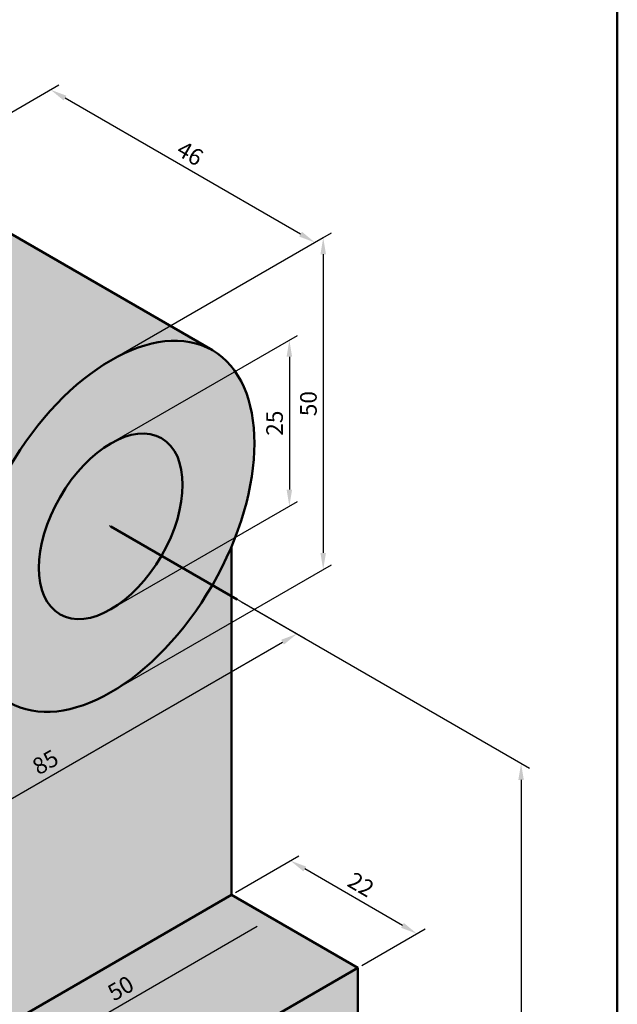
# Model space of a CAD drawing. Units: millimetres. Extents: x 1466 to 1886, y 5011 to 5605.
# Tile 3 of 4: x 1796 to 1886, y 5146 to 5295. Entities that reach past the tile are written whole.
import ezdxf

# ---------------------------------------------------------------- set-up
doc = ezdxf.new("R2010")
doc.units = ezdxf.units.MM
for name, color, linetype, lineweight in [('M-DIMS', 2, 'Continuous', 25), ('M-HATC', 252, 'Continuous', 18), ('M-OUTL', 7, 'Continuous', 50), ('M-TTLB', 7, 'Continuous', 50)]:
    doc.layers.add(name, color=color, linetype=linetype, lineweight=lineweight)
doc.styles.get("Standard").update_dxf_attribs({"font": 'arial.ttf'})
doc.dimstyles.new('ISO-25', dxfattribs={"dimtxt": 2.5, "dimasz": 2.5, "dimexe": 1.25, "dimexo": 0.625, "dimtad": 1, "dimtxsty": 'Standard', "dimcen": 2.5, "dimadec": 0, "dimazin": 0, "dimtfac": 1, "dimtmove": 0, "dimatfit": 3, "dimfxl": 1, "dimarcsym": 0})

# ---------------------------------------------------------------- blocks, each defined once
blk = doc.blocks.new('*D1')
at = {"layer": 'Defpoints', "color": 0, "transparency": 16777216}
for p in [(1828.098835256636, 5162.955036981139), (1834.164568784784, 5159.452984095829), (1784.797565067414, 5137.955036981139)]:
    blk.add_point(p, dxfattribs=at)
at = {"layer": 'M-DIMS', "color": 0, "lineweight": -2, "transparency": 16777216}
for p, q in [((1828.723835256636, 5162.594193062894), (1835.414568784784, 5158.731296259342)), ((1793.028362105023, 5135.702984095829), (1831.999505275323, 5158.202984095829)), ((1785.422565067414, 5137.594193062894), (1792.113298595562, 5133.731296259342))]:
    blk.add_line(p, q, dxfattribs=at)
at = {"layer": 'M-DIMS', "color": 0, "transparency": 16777216}
for points in [[(1831.79117194199, 5158.563828014073), (1832.207838608656, 5157.842140177587), (1834.164568784784, 5159.452984095829)], [(1792.82002877169, 5136.063828014073), (1793.236695438357, 5135.342140177587), (1790.863298595562, 5134.45298409583)]]:
    blk.add_solid(points, dxfattribs=at)
at = {"layer": 'M-DIMS', "color": 0, "transparency": 16777216, "insert": (1811.563217455521, 5148.599672917828), "char_height": 2.5, "attachment_point": 5, "rotation": 30.000000000000025}
blk.add_mtext('50', dxfattribs=at)
blk = doc.blocks.new('*D2')
at = {"layer": 'Defpoints', "color": 0, "transparency": 16777216}
for p in [(1836.996725083254, 5168.092236067757), (1828.098835256635, 5162.955036981138), (1847.151394139893, 5151.955036981138)]:
    blk.add_point(p, dxfattribs=at)
at = {"layer": 'M-DIMS', "color": 0, "lineweight": -2, "transparency": 16777216}
for p, q in [((1828.723835256635, 5163.315880899382), (1838.246725083253, 5168.813923904242)), ((1853.88422045705, 5158.342236067756), (1839.161788592715, 5166.842236067756)), ((1847.776394139893, 5152.315880899382), (1857.299283966511, 5157.813923904242))]:
    blk.add_line(p, q, dxfattribs=at)
at = {"layer": 'M-DIMS', "color": 0, "transparency": 16777216}
for points in [[(1839.370121926048, 5167.203079985999), (1838.953455259381, 5166.481392149512), (1836.996725083254, 5168.092236067757)], [(1854.092553790384, 5158.703079986), (1853.675887123717, 5157.981392149512), (1856.049283966511, 5157.092236067756)]]:
    blk.add_solid(points, dxfattribs=at)
at = {"layer": 'M-DIMS', "color": 0, "transparency": 16777216, "insert": (1847.463062505783, 5164.220464252736), "char_height": 2.5, "attachment_point": 5, "rotation": 330}
blk.add_mtext('22', dxfattribs=at)
blk = doc.blocks.new('*D14')
at = {"layer": 'Defpoints', "color": 0, "transparency": 16777216}
for p in [(1828.964860660421, 5207.455036981141), (1828.964860660421, 5097.45503698114), (1871.761163806512, 5072.74657983943)]:
    blk.add_point(p, dxfattribs=at)
at = {"layer": 'M-DIMS', "color": 0, "lineweight": -2, "transparency": 16777216}
for p, q in [((1829.589860660421, 5207.094193062896), (1873.011163806512, 5182.024892002942)), ((1871.761163806512, 5180.24657983943), (1871.761163806512, 5075.246579839429)), ((1829.589860660421, 5097.094193062897), (1873.011163806512, 5072.024892002943))]:
    blk.add_line(p, q, dxfattribs=at)
at = {"layer": 'M-DIMS', "color": 0, "transparency": 16777216}
for points in [[(1871.344497139845, 5180.24657983943), (1872.177830473179, 5180.24657983943), (1871.761163806512, 5182.74657983943)], [(1871.344497139845, 5075.246579839429), (1872.177830473179, 5075.246579839429), (1871.761163806512, 5072.74657983943)]]:
    blk.add_solid(points, dxfattribs=at)
at = {"layer": 'M-DIMS', "color": 0, "transparency": 16777216, "insert": (1869.859731337209, 5127.746579839429), "char_height": 2.5, "attachment_point": 5, "rotation": 90}
blk.add_mtext('110', dxfattribs=at)
blk = doc.blocks.new('*D21')
at = {"layer": 'Defpoints', "color": 0, "transparency": 16777216}
for p in [(1809.912301777163, 5243.455036981141), (1841.931646665891, 5211.941414371921), (1809.912301777163, 5193.45503698114)]:
    blk.add_point(p, dxfattribs=at)
at = {"layer": 'M-DIMS', "color": 0, "lineweight": -2, "transparency": 16777216}
for p, q in [((1810.537301777164, 5243.815880899385), (1843.181646665891, 5262.66310220841)), ((1841.931646665891, 5259.441414371924), (1841.931646665891, 5214.441414371922)), ((1810.537301777164, 5193.815880899383), (1843.181646665891, 5212.663102208408))]:
    blk.add_line(p, q, dxfattribs=at)
at = {"layer": 'M-DIMS', "color": 0, "transparency": 16777216}
for points in [[(1841.514979999224, 5259.441414371924), (1842.348313332558, 5259.441414371924), (1841.931646665891, 5261.941414371923)], [(1841.514979999224, 5214.441414371922), (1842.348313332558, 5214.441414371922), (1841.931646665891, 5211.941414371921)]]:
    blk.add_solid(points, dxfattribs=at)
at = {"layer": 'M-DIMS', "color": 0, "transparency": 16777216, "insert": (1840.030214196588, 5236.941414371921), "char_height": 2.5, "attachment_point": 5, "rotation": 90}
blk.add_mtext('50', dxfattribs=at)
blk = doc.blocks.new('*D22')
at = {"layer": 'Defpoints', "color": 0, "transparency": 16777216}
for p in [(1809.912301777163, 5230.95503698114), (1836.827511146369, 5221.494540355745), (1809.912301777163, 5205.955036981141)]:
    blk.add_point(p, dxfattribs=at)
at = {"layer": 'M-DIMS', "color": 0, "lineweight": -2, "transparency": 16777216}
for p, q in [((1810.537301777164, 5231.315880899384), (1838.077511146369, 5247.216228192232)), ((1836.827511146369, 5243.994540355746), (1836.827511146369, 5223.994540355746)), ((1810.537301777164, 5206.315880899384), (1838.077511146369, 5222.216228192233))]:
    blk.add_line(p, q, dxfattribs=at)
at = {"layer": 'M-DIMS', "color": 0, "transparency": 16777216}
for points in [[(1836.410844479702, 5243.994540355746), (1837.244177813035, 5243.994540355746), (1836.827511146369, 5246.494540355746)], [(1836.410844479702, 5223.994540355746), (1837.244177813035, 5223.994540355746), (1836.827511146369, 5221.494540355745)]]:
    blk.add_solid(points, dxfattribs=at)
at = {"layer": 'M-DIMS', "color": 0, "transparency": 16777216, "insert": (1834.926078677066, 5233.994540355745), "char_height": 2.5, "attachment_point": 5, "rotation": 90}
blk.add_mtext('25', dxfattribs=at)
blk = doc.blocks.new('*D24')
at = {"layer": 'Defpoints', "color": 0, "transparency": 16777216}
for p in [(1809.046276373379, 5218.955036981139), (1837.969099370778, 5202.256437337866), (1735.434117051702, 5176.455036981138)]:
    blk.add_point(p, dxfattribs=at)
at = {"layer": 'M-DIMS', "color": 0, "lineweight": -2, "transparency": 16777216}
for p, q in [((1809.671276373379, 5218.594193062894), (1839.219099370778, 5201.534749501379)), ((1766.522003558562, 5161.006437337866), (1835.804035861317, 5201.006437337866)), ((1736.059117051701, 5176.094193062894), (1765.606940049101, 5159.03474950138))]:
    blk.add_line(p, q, dxfattribs=at)
at = {"layer": 'M-DIMS', "color": 0, "transparency": 16777216}
for points in [[(1835.595702527983, 5201.367281256109), (1836.01236919465, 5200.645593419623), (1837.969099370778, 5202.256437337866)], [(1766.313670225229, 5161.367281256109), (1766.730336891895, 5160.645593419623), (1764.356940049101, 5159.756437337867)]]:
    blk.add_solid(points, dxfattribs=at)
at = {"layer": 'M-DIMS', "color": 0, "transparency": 16777216, "insert": (1800.212303475287, 5182.653126159864), "char_height": 2.5, "attachment_point": 5, "rotation": 29.99999999999997}
blk.add_mtext('85', dxfattribs=at)
blk = doc.blocks.new('*D25')
at = {"layer": 'Defpoints', "color": 0, "transparency": 16777216}
for p in [(1800.844478091805, 5284.219726535433), (1770.07513320308, 5266.455036981138), (1809.912301777163, 5243.45503698114)]:
    blk.add_point(p, dxfattribs=at)
at = {"layer": 'M-DIMS', "color": 0, "lineweight": -2, "transparency": 16777216}
for p, q in [((1770.70013320308, 5266.815880899383), (1802.094478091805, 5284.941414371921)), ((1838.516583156427, 5262.469726535435), (1803.009541601266, 5282.969726535434)), ((1810.537301777163, 5243.815880899384), (1841.931646665887, 5261.941414371922))]:
    blk.add_line(p, q, dxfattribs=at)
at = {"layer": 'M-DIMS', "color": 0, "transparency": 16777216}
for points in [[(1803.2178749346, 5283.330570453678), (1802.801208267933, 5282.608882617189), (1800.844478091805, 5284.219726535433)], [(1838.72491648976, 5262.830570453679), (1838.308249823093, 5262.108882617191), (1840.681646665888, 5261.219726535435)]]:
    blk.add_solid(points, dxfattribs=at)
at = {"layer": 'M-DIMS', "color": 0, "transparency": 16777216, "insert": (1821.713778613498, 5274.366415357433), "char_height": 2.5, "attachment_point": 5, "rotation": 330.0000000000001}
blk.add_mtext('46', dxfattribs=at)

msp = doc.modelspace()

# ---------------------------------------------------------------- hatches: boundary and pattern name
at = {"layer": 'M-HATC'}
h = msp.add_hatch(color=256, dxfattribs=at)
h.dxf.hatch_style = 1
edge = h.paths.add_edge_path()
edge.add_line((1722.443735994935, 5219.955036981139), (1738.032193263055, 5210.955036981139))
edge.add_line((1738.032193263055, 5210.955036981139), (1722.443735994935, 5201.955036981138))
edge.add_line((1722.443735994935, 5201.955036981138), (1732.836040840348, 5195.955036981139))
edge.add_line((1732.836040840348, 5195.955036981139), (1758.816802953881, 5210.955036981139))
edge.add_line((1758.816802953881, 5210.955036981139), (1748.424498108468, 5216.955036981139))
edge.add_line((1748.424498108468, 5216.955036981139), (1732.836040840348, 5225.955036981138))
edge.add_line((1732.836040840348, 5225.955036981138), (1722.443735994935, 5231.955036981139))
edge.add_line((1722.443735994935, 5231.955036981139), (1712.051431149521, 5225.955036981138))
edge.add_line((1712.051431149521, 5225.955036981138), (1702.481741639855, 5220.429974166671))
edge.add_ellipse((1693.864897670048, 5200.455036981139), major_axis=(-11.02270384252446, -19.0918830920367), ratio=0.5773502691896324, start_angle=186.6654644117269, end_angle=360)
edge.add_line((1682.842193827524, 5181.363153889102), (1695.83257488429, 5173.863153889102))
edge.add_ellipse((1706.855278726814, 5192.955036981139), major_axis=(-11.02270384252446, -19.09188309203669), ratio=0.5773502691896325, start_angle=270, end_angle=359.9999999999998, ccw=False)
edge.add_ellipse((1706.855278726814, 5192.955036981139), major_axis=(-11.02270384252446, -19.09188309203669), ratio=0.5773502691896325, start_angle=210.0000000000012, end_angle=270, ccw=False)
edge.add_line((1706.855278726813, 5210.955036981138), (1722.443735994935, 5219.955036981139))
edge = h.paths.add_edge_path(flags=17)
edge.add_ellipse((1735.434117051701, 5176.455036981138), major_axis=(-11.02270384252446, -19.0918830920367), ratio=0.5773502691896324, start_angle=183.919715644874, end_angle=270, ccw=False)
edge.add_ellipse((1732.836040840348, 5177.955036981138), major_axis=(-11.02270384252446, -19.0918830920367), ratio=0.5773502691896323, start_angle=176.0802843551266, end_angle=210.0000000000004)
edge.add_line((1732.836040840348, 5195.955036981139), (1722.443735994935, 5201.955036981138))
edge.add_ellipse((1722.443735994935, 5183.955036981139), major_axis=(-11.02270384252446, -19.0918830920367), ratio=0.5773502691896323, start_angle=210.0000000000004, end_angle=266.235889459397)
edge.add_ellipse((1706.855278726814, 5192.955036981139), major_axis=(-4.592793267718468, -7.954951288348655), ratio=0.5773502691896232, start_angle=90, end_angle=99.00326933995552, ccw=False)
edge.add_line((1711.448071994533, 5190.303386551689), (1724.411413209177, 5182.818998011818))
edge = h.paths.add_edge_path()
edge.add_line((1724.411413209177, 5182.818998011818), (1711.448071994533, 5190.303386551689))
edge.add_ellipse((1706.855278726814, 5192.955036981139), major_axis=(-4.592793267718468, -7.954951288348655), ratio=0.5773502691896232, start_angle=80.9967306600526, end_angle=90, ccw=False)
edge.add_ellipse((1722.443735994935, 5183.955036981139), major_axis=(-11.02270384252446, -19.0918830920367), ratio=0.5773502691896323, start_angle=273.764110540599, end_angle=329.9999999999981)
edge.add_ellipse((1722.443735994935, 5183.955036981139), major_axis=(-11.02270384252446, -19.0918830920367), ratio=0.5773502691896323, start_angle=329.9999999999981, end_angle=360)
edge.add_line((1711.42103215241, 5164.863153889102), (1724.411413209177, 5157.363153889102))
edge.add_ellipse((1735.434117051701, 5176.455036981138), major_axis=(-11.02270384252446, -19.0918830920367), ratio=0.5773502691896324, start_angle=270, end_angle=360, ccw=False)
edge = h.paths.add_edge_path(flags=17)
edge.add_line((1758.816802953881, 5210.955036981139), (1732.836040840348, 5195.955036981139))
edge.add_ellipse((1732.836040840348, 5177.955036981138), major_axis=(-11.02270384252446, -19.0918830920367), ratio=0.5773502691896323, start_angle=176.0802843551266, end_angle=210.0000000000005, ccw=False)
edge.add_ellipse((1735.434117051701, 5176.455036981138), major_axis=(-11.02270384252446, -19.0918830920367), ratio=0.5773502691896324, start_angle=70.6800531201103, end_angle=183.919715644874, ccw=False)
edge.add_line((1744.050961021509, 5166.429974166671), (1758.816802953881, 5174.955036981138))
edge.add_line((1758.816802953881, 5174.955036981138), (1758.816802953881, 5210.955036981139))
edge = h.paths.add_edge_path(flags=17)
edge.add_ellipse((1797.78794612418, 5225.455036981139), major_axis=(-15.30931089239438, -26.5165042944958), ratio=0.5773502691896226, start_angle=218.6849191088683, end_angle=329.99999999999915, ccw=False)
edge.add_line((1794.323844509042, 5248.132962339644), (1748.424498108468, 5216.955036981139))
edge.add_line((1748.424498108468, 5216.955036981139), (1758.816802953881, 5210.955036981139))
edge.add_line((1758.816802953881, 5210.955036981139), (1758.816802953881, 5186.955036981139))
edge.add_line((1758.816802953881, 5186.955036981139), (1776.13731102957, 5196.955036981139))
edge.add_line((1776.13731102957, 5196.955036981139), (1776.13731102957, 5212.955036981139))
edge = h.paths.add_edge_path()
edge.add_ellipse((1797.78794612418, 5225.455036981139), major_axis=(-15.30931089239438, -26.5165042944958), ratio=0.5773502691896226, start_angle=218.6849191088682, end_angle=329.9999999999991)
edge.add_line((1776.13731102957, 5212.955036981139), (1776.13731102957, 5196.955036981139))
edge.add_line((1776.13731102957, 5196.955036981139), (1769.209107799294, 5192.955036981139))
edge.add_line((1769.209107799294, 5192.955036981139), (1769.209107799294, 5146.955036981139))
edge.add_line((1769.209107799294, 5146.955036981139), (1784.797565067414, 5137.955036981139))
edge.add_line((1784.797565067414, 5137.955036981139), (1784.797565067414, 5155.95503698114))
edge.add_line((1784.797565067414, 5155.95503698114), (1784.797565067414, 5207.955036981145))
edge.add_ellipse((1806.448200162025, 5220.455036981139), major_axis=(-15.30931089239438, -26.5165042944958), ratio=0.5773502691896227, start_angle=329.9999999999989, end_angle=363.7613167964908)
edge.add_ellipse((1809.912301777163, 5218.455036981139), major_axis=(-15.30931089239438, -26.5165042944958), ratio=0.5773502691896226, start_angle=179.9999999999992, end_angle=356.23868320351306, ccw=False)
edge.add_line((1825.221612669557, 5244.971541275634), (1785.384444095473, 5267.971541275635))
edge.add_ellipse((1770.075133203079, 5241.455036981139), major_axis=(-15.30931089239438, -26.5165042944958), ratio=0.5773502691896226, start_angle=540, end_angle=311.5164128123438)
edge.add_line((1749.475859885243, 5237.257922029503), (1732.836040840348, 5225.955036981138))
edge.add_line((1732.836040840348, 5225.955036981138), (1748.424498108468, 5216.955036981139))
edge.add_line((1748.424498108468, 5216.955036981139), (1794.323844509042, 5248.132962339644))
edge = h.paths.add_edge_path()
edge.add_line((1828.098835256636, 5207.955036981139), (1825.221612669557, 5209.616202216307))
edge.add_ellipse((1809.912301777163, 5218.455036981139), major_axis=(-15.30931089239438, -26.5165042944958), ratio=0.5773502691896226, start_angle=356.23868320351306, end_angle=449.99999999999966, ccw=False)
edge.add_ellipse((1806.448200162025, 5220.455036981139), major_axis=(-15.30931089239438, -26.5165042944958), ratio=0.5773502691896227, start_angle=329.99999999999886, end_angle=363.76131679649075, ccw=False)
edge.add_line((1784.797565067414, 5207.955036981145), (1784.797565067414, 5155.95503698114))
edge.add_line((1784.797565067414, 5155.95503698114), (1784.797565067414, 5137.955036981139))
edge.add_line((1784.797565067414, 5137.955036981139), (1828.098835256636, 5162.955036981139))
edge.add_line((1828.098835256636, 5162.955036981139), (1828.098835256636, 5207.955036981139))
edge = h.paths.add_edge_path()
edge.add_ellipse((1809.912301777163, 5218.455036981139), major_axis=(-15.30931089239438, -26.5165042944958), ratio=0.5773502691896226, start_angle=89.99999999999972, end_angle=110.43480323036249, ccw=False)
edge.add_line((1825.221612669557, 5209.616202216307), (1828.098835256636, 5207.955036981139))
edge.add_line((1828.098835256636, 5207.955036981139), (1828.098835256636, 5215.390377014889))
h.paths.add_polyline_path([(1769.209107799294, 5168.955036981138), (1750.156548916036, 5157.955036981139), (1769.209107799294, 5146.955036981139)], flags=17)
h.paths.add_polyline_path([(1847.151394139893, 5151.955036981139), (1828.098835256636, 5162.955036981139), (1784.797565067414, 5137.955036981139), (1803.850123950671, 5126.955036981138)])
edge = h.paths.add_edge_path()
edge.add_ellipse((1825.500759045282, 5099.455036981138), major_axis=(-17.14642819948207, -29.69848480983509), ratio=0.577350269189623, start_angle=176.6451013603207, end_angle=299.71017051362753, ccw=False)
edge.add_ellipse((1828.96486066042, 5097.455036981139), major_axis=(-17.14642819948207, -29.69848480983509), ratio=0.577350269189623, start_angle=177.9252840891673, end_angle=183.3548986396804, ccw=False)
edge.add_line((1847.151394139893, 5126.47529615859), (1847.151394139893, 5151.955036981139))
edge.add_line((1847.151394139893, 5151.955036981139), (1804.3764033923, 5127.258884558432))
edge.add_ellipse((1813.3764033923, 5106.455036981138), major_axis=(-17.14642819948207, -29.69848480983509), ratio=0.577350269189623, start_angle=233.3939017938641, end_angle=235.1951901217888)
edge.add_line((1803.850123950671, 5126.703823360306), (1803.850123950671, 5099.564557194057))
edge = h.paths.add_edge_path()
edge.add_ellipse((1828.96486066042, 5097.455036981139), major_axis=(-17.14642819948207, -29.69848480983509), ratio=0.577350269189623, start_angle=183.3548986396804, end_angle=360, ccw=False)
edge.add_ellipse((1825.500759045282, 5099.455036981138), major_axis=(-17.14642819948207, -29.69848480983509), ratio=0.577350269189623, start_angle=176.6451013603206, end_angle=299.7101705136275)
edge.add_line((1803.850123950671, 5099.564557194057), (1803.850123950671, 5126.703823360306))
edge.add_line((1803.850123950671, 5126.703823360306), (1803.850123950671, 5126.955036981138))
edge.add_line((1803.850123950671, 5126.955036981138), (1784.797565067414, 5137.955036981139))
edge.add_line((1784.797565067414, 5137.955036981139), (1769.209107799294, 5146.955036981139))
edge.add_line((1769.209107799294, 5146.955036981139), (1750.156548916036, 5157.955036981139))
edge.add_line((1750.156548916036, 5157.955036981139), (1750.156548916036, 5139.867928007788))
edge.add_ellipse((1769.165624306577, 5133.458728431643), major_axis=(-17.14642819948207, -29.69848480983509), ratio=0.577350269189623, start_angle=281.3676816797435, end_angle=360)
edge.add_line((1752.019196107095, 5103.760243621808), (1765.421555363387, 5094.680341464254))
edge.add_ellipse((1783.931539663629, 5123.455036981138), major_axis=(-17.14642819948207, -29.69848480983509), ratio=0.577350269189623, start_angle=299.7101705136324, end_angle=357.2479180547133, ccw=False)
edge.add_line((1762.280904569018, 5123.564557194055), (1762.280904569018, 5138.955036981139))
edge.add_line((1762.280904569018, 5138.955036981139), (1784.797565067414, 5125.955036981139))
edge.add_line((1784.797565067414, 5125.955036981139), (1791.725768297689, 5121.955036981138))
edge.add_line((1791.725768297689, 5121.955036981138), (1791.725768297689, 5106.564557194055))
edge.add_ellipse((1813.3764033923, 5106.455036981138), major_axis=(-17.14642819948207, -29.69848480983509), ratio=0.577350269189623, start_angle=299.7101705136277, end_angle=315.9583021122638)
edge.add_ellipse((1813.3764033923, 5106.455036981138), major_axis=(-17.14642819948207, -29.69848480983509), ratio=0.577350269189623, start_angle=315.9583021122638, end_angle=360)
edge.add_line((1796.229975192818, 5076.756552171303), (1811.818432460938, 5067.756552171303))
h = msp.add_hatch(color=256, dxfattribs=at)
h.dxf.hatch_style = 1
edge = h.paths.add_edge_path()
edge.add_ellipse((1809.912301777163, 5218.455036981139), major_axis=(-7.654655446197786, -13.25825214724756), ratio=0.5773502691896373, start_angle=90, end_angle=360, ccw=False)
edge.add_line((1817.56695722336, 5214.035619598722), (1825.221612669557, 5209.616202216307))
edge.add_ellipse((1809.912301777163, 5218.455036981139), major_axis=(-15.30931089239438, -26.5165042944958), ratio=0.5773502691896226, start_angle=89.99999999999962, end_angle=110.4348032303624)
edge.add_ellipse((1809.912301777163, 5218.455036981139), major_axis=(-15.30931089239438, -26.5165042944958), ratio=0.5773502691896226, start_angle=110.4348032303624, end_angle=179.9999999999991)
edge.add_ellipse((1809.912301777163, 5218.455036981139), major_axis=(-15.30931089239438, -26.5165042944958), ratio=0.5773502691896226, start_angle=179.9999999999991, end_angle=356.2386832035131)
edge.add_ellipse((1809.912301777163, 5218.455036981139), major_axis=(-15.30931089239438, -26.5165042944958), ratio=0.5773502691896226, start_angle=356.2386832035131, end_angle=449.9999999999996)
edge.add_line((1825.221612669557, 5209.616202216307), (1817.56695722336, 5214.035619598722))
edge.add_ellipse((1809.912301777163, 5218.455036981139), major_axis=(-7.654655446197786, -13.25825214724756), ratio=0.5773502691896373, start_angle=0, end_angle=90, ccw=False)
edge = h.paths.add_edge_path()
edge.add_ellipse((1735.434117051701, 5176.455036981138), major_axis=(-11.02270384252446, -19.0918830920367), ratio=0.5773502691896324, start_angle=70.68005312011024, end_angle=183.9197156448739)
edge.add_ellipse((1735.434117051701, 5176.455036981138), major_axis=(-11.02270384252446, -19.0918830920367), ratio=0.5773502691896324, start_angle=183.9197156448739, end_angle=270)
edge.add_line((1724.411413209177, 5182.818998011818), (1730.841323783983, 5179.106687410587))
edge.add_ellipse((1735.434117051701, 5176.455036981138), major_axis=(-4.592793267718468, -7.954951288348655), ratio=0.5773502691896234, start_angle=0, end_angle=270, ccw=False)
edge.add_ellipse((1735.434117051701, 5176.455036981138), major_axis=(-4.592793267718468, -7.954951288348655), ratio=0.5773502691896234, start_angle=270, end_angle=360, ccw=False)
edge.add_line((1730.841323783983, 5179.106687410587), (1724.411413209177, 5182.818998011818))
edge.add_ellipse((1735.434117051701, 5176.455036981138), major_axis=(-11.02270384252446, -19.0918830920367), ratio=0.5773502691896324, start_angle=270, end_angle=360)
edge.add_ellipse((1735.434117051701, 5176.455036981138), major_axis=(-11.02270384252446, -19.0918830920367), ratio=0.5773502691896324, start_angle=0, end_angle=70.68005312011029)
edge = h.paths.add_edge_path()
edge.add_line((1722.443735994935, 5219.955036981139), (1706.855278726813, 5210.955036981138))
edge.add_ellipse((1706.855278726814, 5192.955036981139), major_axis=(-11.02270384252446, -19.09188309203669), ratio=0.5773502691896325, start_angle=210.0000000000012, end_angle=270)
edge.add_line((1695.83257488429, 5199.318998011818), (1702.262485459096, 5195.606687410588))
edge.add_ellipse((1706.855278726814, 5192.955036981139), major_axis=(-4.592793267718468, -7.954951288348655), ratio=0.5773502691896232, start_angle=99.00326933995552, end_angle=270, ccw=False)
edge.add_ellipse((1722.443735994935, 5183.955036981139), major_axis=(-11.02270384252446, -19.0918830920367), ratio=0.5773502691896323, start_angle=210.0000000000005, end_angle=266.2358894593971, ccw=False)
edge.add_line((1722.443735994935, 5201.955036981138), (1722.443735994935, 5219.955036981139))
edge = h.paths.add_edge_path()
edge.add_ellipse((1722.443735994935, 5183.955036981139), major_axis=(-11.02270384252446, -19.0918830920367), ratio=0.5773502691896323, start_angle=273.76411054059906, end_angle=329.9999999999982, ccw=False)
edge.add_ellipse((1706.855278726814, 5192.955036981139), major_axis=(-4.592793267718468, -7.954951288348655), ratio=0.5773502691896232, start_angle=270, end_angle=440.9967306600526, ccw=False)
edge.add_line((1702.262485459096, 5195.606687410588), (1695.83257488429, 5199.318998011818))
edge.add_ellipse((1706.855278726814, 5192.955036981139), major_axis=(-11.02270384252446, -19.09188309203669), ratio=0.5773502691896325, start_angle=270, end_angle=359.9999999999997)
edge.add_ellipse((1706.855278726814, 5192.955036981139), major_axis=(-11.02270384252446, -19.09188309203669), ratio=0.5773502691896325, start_angle=359.9999999999997, end_angle=390.0000000000012)
edge = h.paths.add_edge_path()
edge.add_ellipse((1828.96486066042, 5097.455036981139), major_axis=(-17.14642819948207, -29.69848480983509), ratio=0.577350269189623, start_angle=0, end_angle=177.9252840891672)
edge.add_ellipse((1828.96486066042, 5097.455036981139), major_axis=(-17.14642819948207, -29.69848480983509), ratio=0.577350269189623, start_angle=177.9252840891672, end_angle=183.3548986396804)
edge.add_ellipse((1828.96486066042, 5097.455036981139), major_axis=(-17.14642819948207, -29.69848480983509), ratio=0.577350269189623, start_angle=183.3548986396804, end_angle=360)
edge = h.paths.add_edge_path(flags=16)
edge.add_ellipse((1828.96486066042, 5097.455036981139), major_axis=(-9.79795897113284, -16.97056274847708), ratio=0.5773502691896234, start_angle=217.1598249325803, end_angle=322.84017506741907, ccw=False)
edge.add_ellipse((1828.96486066042, 5097.455036981139), major_axis=(-9.79795897113284, -16.97056274847708), ratio=0.5773502691896234, start_angle=322.84017506741907, end_angle=577.1598249325802, ccw=False)
edge = h.paths.add_edge_path()
edge.add_line((1791.725768297689, 5106.564557194055), (1791.725768297689, 5114.726280425816))
edge.add_ellipse((1783.931539663629, 5123.455036981138), major_axis=(-9.797958971132836, -16.97056274847707), ratio=0.5773502691896235, start_angle=322.84017506742066, end_angle=431.7628416390562, ccw=False)
edge.add_ellipse((1783.931539663629, 5123.455036981138), major_axis=(-9.797958971132836, -16.97056274847707), ratio=0.5773502691896235, start_angle=256.9555772654587, end_angle=322.84017506742066, ccw=False)
edge.add_line((1775.519115469529, 5131.31195235414), (1762.280904569018, 5138.955036981139))
edge.add_line((1762.280904569018, 5138.955036981139), (1762.280904569018, 5123.564557194055))
edge.add_ellipse((1783.931539663629, 5123.455036981138), major_axis=(-17.14642819948207, -29.69848480983509), ratio=0.577350269189623, start_angle=299.7101705136324, end_angle=357.2479180547133)
edge.add_line((1765.421555363387, 5094.680341464254), (1766.785111464145, 5093.756552171305))
edge.add_ellipse((1783.931539663629, 5123.455036981138), major_axis=(-17.14642819948207, -29.69848480983509), ratio=0.577350269189623, start_angle=359.9999999999943, end_angle=404.0416978877337)
edge.add_ellipse((1813.3764033923, 5106.455036981138), major_axis=(-17.14642819948207, -29.69848480983509), ratio=0.577350269189623, start_angle=299.71017051362776, end_angle=315.95830211226377, ccw=False)
h = msp.add_hatch(color=256, dxfattribs=at)
h.dxf.hatch_style = 1
edge = h.paths.add_edge_path()
edge.add_ellipse((1735.434117051701, 5176.455036981138), major_axis=(-4.592793267718468, -7.954951288348655), ratio=0.5773502691896234, start_angle=0, end_angle=270)
edge.add_ellipse((1735.434117051701, 5176.455036981138), major_axis=(-4.592793267718468, -7.954951288348655), ratio=0.5773502691896234, start_angle=270, end_angle=360)
edge = h.paths.add_edge_path()
edge.add_ellipse((1809.912301777163, 5218.455036981139), major_axis=(-7.654655446197786, -13.25825214724756), ratio=0.5773502691896373, start_angle=90.00000000000003, end_angle=360)
edge.add_ellipse((1809.912301777163, 5218.455036981139), major_axis=(-7.654655446197786, -13.25825214724756), ratio=0.5773502691896373, start_angle=0, end_angle=90)
edge = h.paths.add_edge_path()
edge.add_ellipse((1706.855278726814, 5192.955036981139), major_axis=(-4.592793267718468, -7.954951288348655), ratio=0.5773502691896232, start_angle=99.00326933995547, end_angle=270)
edge.add_line((1702.262485459096, 5195.606687410588), (1711.42103215241, 5190.318998011818))
edge.add_ellipse((1722.443735994935, 5183.955036981139), major_axis=(-11.02270384252446, -19.0918830920367), ratio=0.5773502691896323, start_angle=266.2358894593971, end_angle=270, ccw=False)
edge = h.paths.add_edge_path()
edge.add_ellipse((1722.443735994935, 5183.955036981139), major_axis=(-11.02270384252446, -19.0918830920367), ratio=0.5773502691896323, start_angle=270, end_angle=273.76411054059906, ccw=False)
edge.add_line((1711.42103215241, 5190.318998011818), (1702.262485459096, 5195.606687410588))
edge.add_ellipse((1706.855278726814, 5192.955036981139), major_axis=(-4.592793267718468, -7.954951288348655), ratio=0.5773502691896232, start_angle=270, end_angle=440.9967306600525)
edge = h.paths.add_edge_path()
edge.add_ellipse((1828.96486066042, 5097.455036981139), major_axis=(-9.79795897113284, -16.97056274847708), ratio=0.5773502691896234, start_angle=322.840175067419, end_angle=217.1598249325803)
edge.add_ellipse((1813.3764033923, 5106.455036981138), major_axis=(-9.797958971132836, -16.97056274847707), ratio=0.5773502691896235, start_angle=397.1598249325802, end_angle=502.8401750674186, ccw=False)
edge = h.paths.add_edge_path()
edge.add_line((1791.725768297689, 5121.955036981138), (1784.797565067414, 5125.955036981139))
edge.add_line((1784.797565067414, 5125.955036981139), (1779.353582800964, 5129.098121608137))
edge.add_ellipse((1768.343082395509, 5132.455036981139), major_axis=(-9.797958971132836, -16.97056274847707), ratio=0.5773502691896235, start_angle=397.1598249325797, end_angle=463.0444227345428, ccw=False)
edge.add_ellipse((1783.931539663629, 5123.455036981138), major_axis=(-9.797958971132836, -16.97056274847707), ratio=0.5773502691896235, start_angle=322.8401750674207, end_angle=431.7628416390561)
edge.add_line((1791.725768297689, 5114.726280425816), (1791.725768297689, 5121.955036981138))

# ---------------------------------------------------------------- linework, layer by layer
at = {"layer": 'M-OUTL'}
for p, q in [((1825.221612669557, 5244.971541275634), (1785.384444095473, 5267.971541275635)), ((1828.96486066042, 5207.455036981139), (1809.912301777163, 5218.455036981139)), ((1828.098835256636, 5215.390377014887), (1828.098835256636, 5162.955036981139)), ((1784.797565067414, 5137.955036981139), (1828.098835256636, 5162.955036981139)), ((1828.098835256636, 5162.955036981139), (1847.151394139893, 5151.955036981139)), ((1847.151394139893, 5151.955036981139), (1803.850123950671, 5126.955036981138)), ((1847.151394139893, 5151.955036981139), (1847.151394139893, 5126.47529615859))]:
    msp.add_line(p, q, dxfattribs=at)
for major_axis, ratio in [((-15.30931089239438, -26.5165042944958), 0.5773502691896226), ((-7.654655446197784, -13.25825214724756), 0.5773502691896374)]:
    msp.add_ellipse((1809.912301777163, 5218.455036981139), major_axis=major_axis, ratio=ratio, dxfattribs=at)
at = {"layer": 'M-TTLB'}
msp.add_lwpolyline([(1466.267100225985, 5604.631473972534), (1886.267100225985, 5604.631473972534), (1886.267100225985, 5010.631473972534), (1466.267100225985, 5010.631473972534)], close=True, dxfattribs=at)

# ---------------------------------------------------------------- dimensions: what is measured, and where the dimension line sits
at = {"layer": 'M-DIMS'}
for p1, p2, distance, picture, middle in [((1809.912301777163, 5243.455036981139), (1770.07513320308, 5266.455036981138), -30.769344888726597, '*D25', (1821.713778613498, 5274.366415357433)), ((1809.912301777163, 5243.455036981139), (1809.912301777163, 5193.455036981138), 32.01934488872803, '*D21', (1840.030214196588, 5236.941414371921)), ((1809.912301777163, 5230.955036981139), (1809.912301777163, 5205.955036981139), 26.915209369205968, '*D22', (1834.926078677066, 5233.994540355745)), ((1735.434117051701, 5176.455036981138), (1809.046276373379, 5218.955036981139), -28.922822997399088, '*D24', (1800.212303475287, 5182.653126159864)), ((1828.96486066042, 5207.455036981139), (1828.96486066042, 5097.455036981139), 42.79630314609198, '*D14', (1869.859731337209, 5127.746579839429)), ((1847.151394139893, 5151.955036981139), (1828.098835256636, 5162.955036981139), -8.897889826618677, '*D2', (1847.463062505783, 5164.220464252736)), ((1784.797565067414, 5137.955036981139), (1828.098835256636, 5162.955036981139), -6.065733528148409, '*D1', (1811.563217455521, 5148.599672917828))]:
    dim = msp.add_aligned_dim(p1=p1, p2=p2, distance=distance, dimstyle='ISO-25', override={"dimclrd": 0, "dimclre": 0, "dimclrt": 0}, dxfattribs=at)
    dim.commit()
    dim.dimension.update_dxf_attribs({"geometry": picture, "text_midpoint": middle})

doc.saveas('drawing.dxf')
